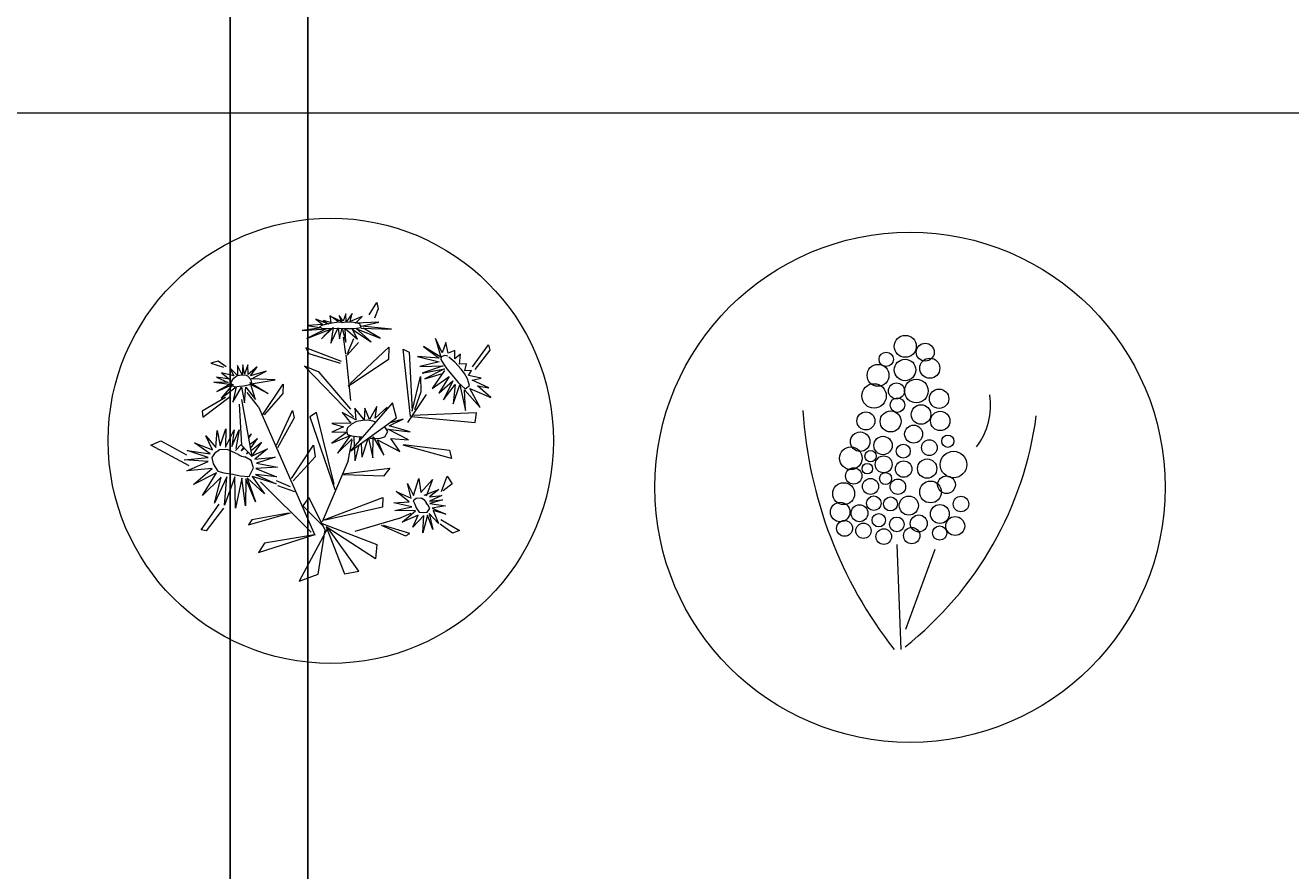
# Model space of a CAD drawing. Units: inches. Extents: x 8049 to 8459, y 820 to 1350.
# Tile 16 of 25: x 8132 to 8165, y 930 to 952. Entities that reach past the tile are written whole.
import ezdxf

# ---------------------------------------------------------------- set-up
doc = ezdxf.new("R2010")
doc.units = ezdxf.units.IN
doc.header["$MEASUREMENT"] = 0
for name, color, linetype, lineweight in [('A-ANNO-DIMS', 2, 'Continuous', 18), ('L-PLNT-BEDS', 94, 'Continuous', 18), ('zelen', 69, 'Continuous', 13)]:
    doc.layers.add(name, color=color, linetype=linetype, lineweight=lineweight)
doc.styles.get("Standard").update_dxf_attribs({"font": 'arial.ttf'})
doc.dimstyles.get("Standard").update_dxf_attribs({"dimtxt": 0.18, "dimasz": 0.18, "dimexe": 0.18, "dimexo": 0.0625, "dimgap": 0.09, "dimtad": 0, "dimtih": 1, "dimtoh": 1, "dimdec": 4, "dimzin": 0, "dimdsep": 46, "dimtxsty": 'Standard', "dimcen": 0.09, "dimadec": 0, "dimazin": 0, "dimtfac": 1, "dimtdec": 4, "dimtofl": 0, "dimtmove": 0, "dimatfit": 3, "dimfxl": 1, "dimtolj": 1, "dimtzin": 0, "dimarcsym": 0})

# ---------------------------------------------------------------- blocks, each defined once
blk = doc.blocks.new('z_07')
for p, q in [((33.4, 283.2), (27.9, 266.9)), ((34.5, 265), (33.4, 283.2)), ((47.8, 284), (34.5, 265)), ((43.1, 265.9), (47.8, 284)), ((85.3, 280.8), (103, 308.6)), ((105.8, 294.2), (97.8, 273.4)), ((103, 308.6), (105.8, 294.2)), ((-17.8, 259.4), (-52, 257.4)), ((-52, 257.4), (-21, 251.8)), ((-33.4, 271.7), (-17.8, 259.4)), ((-5.4, 260.2), (-33.4, 271.7)), ((-17.3, 268.5), (-5.4, 260.2)), ((0.4, 263.9), (-17.3, 268.5)), ((-2, 279), (0.4, 263.9)), ((16.1, 266.2), (-2, 279)), ((6.4, 274.5), (16.1, 266.2)), ((23.4, 266.3), (6.4, 274.5)), ((19, 279.6), (23.4, 266.3)), ((27.9, 266.9), (19, 279.6)), ((70.3, 277.4), (43.1, 265.9)), ((55.3, 262.3), (70.3, 277.4)), ((107.1, 264.9), (55.3, 262.3)), ((68.5, 256.1), (107.1, 264.9)), ((135.2, 249.3), (68.5, 256.1)), ((-21, 251.8), (-63.9, 246.3)), ((-63.9, 246.3), (-10.6, 249.9)), ((-10.6, 249.9), (-53.8, 228)), ((-53.8, 228), (-0.5, 249)), ((-20.7, 227.5), (5.4, 252.6)), ((-0.5, 249), (-20.7, 227.5)), ((5.4, 252.6), (-0.2, 218.2)), ((-0.2, 218.2), (16.1, 251.8)), ((16.1, 251.8), (19.1, 227.4)), ((19.1, 227.4), (25, 251.4)), ((25, 251.4), (33.2, 219.8)), ((33.5, 194.3), (28.4, 231.3)), ((31.7, 250.6), (59.3, 226.6)), ((33.2, 219.8), (31.7, 250.6)), ((37.5, 194.8), (51.1, 228.1)), ((48.1, 248.2), (90.3, 221.2)), ((59.3, 226.6), (48.1, 248.2)), ((57.3, 249.7), (110, 229.2)), ((90.3, 221.2), (57.3, 249.7)), ((67.6, 251), (135.2, 249.3)), ((110, 229.2), (72.3, 251.5)), ((234, 228.4), (245.3, 186.3)), ((248.2, 196), (234, 228.4)), ((-56, 207.7), (-48.9, 194.5)), ((23.9, 176.8), (-56, 207.7)), ((61.7, 219.6), (36.6, 191.4)), ((43.1, 127.7), (129.4, 208.7)), ((129.4, 208.7), (129.1, 181.5)), ((161.2, 204.4), (175.2, 197.9)), ((177.8, 54.5), (161.2, 204.4)), ((175.2, 197.9), (181.3, 66.4)), ((207.2, 210.7), (242, 184.3)), ((245.3, 186.3), (207.2, 210.7)), ((256.8, 219), (248.2, 196)), ((261.8, 195.5), (256.8, 219)), ((276.9, 201.7), (261.8, 195.5)), ((276.6, 182.8), (276.9, 201.7)), ((316.3, 165), (351.8, 213.8)), ((354.7, 202.6), (321.1, 159.3)), ((351.8, 213.8), (354.7, 202.6)), ((-251.2, 177.7), (-267.6, 173.3)), ((-267.6, 173.3), (-239.8, 164.3)), ((-233.4, 165.2), (-251.2, 177.7)), ((-196.5, 169.7), (-197.8, 147.3)), ((-192.3, 148.3), (-196.5, 169.7)), ((-48.9, 194.5), (20.9, 173)), ((33.4, 191.9), (44, 90.1)), ((129.1, 181.5), (39.1, 121.3)), ((193.5, 188), (242.1, 176.2)), ((242, 184.3), (193.5, 188)), ((242.1, 176.2), (198.4, 166.1)), ((246.2, 187.2), (245.4, 181.5)), ((245.4, 181.5), (251.2, 171.8)), ((254.4, 190.4), (246.2, 187.2)), ((251.2, 171.8), (258.8, 160.8)), ((261.3, 189.2), (254.4, 190.4)), ((277.1, 175.7), (263.7, 186.3)), ((289.7, 193.6), (276.6, 182.8)), ((290.7, 160), (277.1, 175.7)), ((287, 171.3), (289.7, 193.6)), ((302.8, 171.8), (287, 171.3)), ((299, 156), (302.8, 171.8)), ((-255.4, 142.2), (-228.7, 129.8)), ((-226, 137.3), (-255.4, 142.2)), ((-243.6, 151.8), (-226, 137.3)), ((-216.2, 145.1), (-243.6, 151.8)), ((-225.7, 163.4), (-216.2, 145.1)), ((-208.5, 145.4), (-225.7, 163.4)), ((-208.7, 144.6), (-219.5, 136.6)), ((-198.7, 146.1), (-208.7, 144.6)), ((-207.9, 168.2), (-208.5, 145.4)), ((-197.8, 147.3), (-207.9, 168.2)), ((-188, 145.4), (-198.7, 146.1)), ((-185.4, 169.2), (-192.3, 148.3)), ((-185.1, 144.1), (-188, 145.4)), ((-184.1, 147.7), (-185.4, 169.2)), ((-179.1, 137.8), (-185.1, 144.1)), ((-164.3, 164.9), (-184.1, 147.7)), ((-179.3, 144.6), (-164.3, 164.9)), ((-144.4, 155), (-179.3, 144.6)), ((-177.3, 138.3), (-144.4, 155)), ((-58.7, 166.4), (50.5, 53.3)), ((-25.8, 153.4), (-58.7, 166.4)), ((44.9, 70.5), (-25.8, 153.4)), ((181.3, 66.4), (199.9, 143.5)), ((198.4, 166.1), (251.1, 167.3)), ((199.9, 143.5), (200.9, 108.9)), ((251.1, 167.3), (203.7, 151)), ((203.7, 151), (254, 160.4)), ((254, 160.4), (209.5, 138.3)), ((209.5, 138.3), (249.1, 150.4)), ((253.9, 156.5), (226.3, 116.7)), ((226.3, 116.7), (263.8, 143.7)), ((263.8, 143.7), (241.3, 106.4)), ((258.8, 160.8), (271.1, 146.1)), ((271.1, 146.1), (284.2, 130.2)), ((298.2, 149.9), (290.7, 160)), ((305.4, 138.6), (298.2, 149.9)), ((314, 156.8), (299, 156)), ((307.2, 145.4), (314, 156.8)), ((335.8, 139.8), (307.2, 145.4)), ((-260.9, 130.5), (-225.2, 126.2)), ((-228.7, 129.8), (-260.9, 130.5)), ((-254.6, 110.2), (-218.2, 126.3)), ((-225.2, 126.2), (-254.6, 110.2)), ((-218.2, 126.3), (-244.5, 95.4)), ((-244.5, 95.4), (-211, 120.2)), ((-219.5, 136.6), (-223.8, 129.5)), ((-223.8, 129.5), (-220.3, 123.5)), ((-220.3, 123.5), (-214.4, 120.6)), ((-211, 120.2), (-218.7, 86)), ((-218.7, 86), (-199, 119.8)), ((-214.4, 120.6), (-204.4, 121.7)), ((-204.4, 121.7), (-194.8, 122.3)), ((-199, 119.8), (-192.3, 84.8)), ((-194.8, 122.3), (-183.9, 124.5)), ((-192.3, 84.8), (-189.8, 119.4)), ((-189.8, 119.4), (-168.3, 91.9)), ((-183.9, 124.5), (-175.3, 127)), ((-179.8, 129.8), (-139.5, 105.2)), ((-168.3, 91.9), (-179.8, 129.8)), ((-177.1, 133.3), (-179.1, 137.8)), ((-177.5, 126.2), (-176.4, 128.6)), ((-139.5, 105.2), (-177.5, 124.5)), ((-124, 136.2), (-177.3, 138.3)), ((-176.4, 128.6), (-177.1, 133.3)), ((-173.3, 127.9), (-124, 136.2)), ((-153, 56.3), (-106.3, 126)), ((-106.3, 126), (-106.9, 105.8)), ((241.3, 106.4), (272.2, 133.8)), ((272.2, 133.8), (251.6, 91.4)), ((251.6, 91.4), (277.6, 125.4)), ((277.6, 125.4), (273.2, 82.7)), ((273.2, 82.7), (288.2, 124.6)), ((284.2, 130.2), (299.9, 116.2)), ((288.2, 124.6), (300.3, 67.6)), ((298.3, 113.8), (333.6, 74.1)), ((300.3, 67.6), (298.3, 113.8)), ((299.9, 116.2), (309.5, 123)), ((309.5, 123), (305.4, 138.6)), ((310, 116.8), (357.4, 96.4)), ((333.6, 74.1), (310, 116.8)), ((315.5, 135.5), (335.8, 139.8)), ((352.4, 118.2), (315.5, 135.5)), ((327.7, 122.6), (352.4, 118.2)), ((357.4, 96.4), (327.7, 122.6)), ((-235.3, 96.4), (-287.1, 65.9)), ((-285.8, 52.5), (-224.8, 98.6)), ((-175.3, -35.1), (-198.7, 92.4)), ((-161, 75.8), (-186.5, 108.1)), ((-106.9, 105.8), (-148.5, 57.6)), ((213, 103.6), (171.4, 40.8)), ((200.9, 108.9), (186.6, 68.8)), ((-287.1, 65.9), (-285.8, 52.5)), ((-204.6, 81.4), (-199.5, -9.8)), ((-161, 75.8), (-35.7, -210.4)), ((-121, -10), (-85.7, 67.7)), ((-85.7, 67.7), (-81.5, 51.1)), ((-32.2, 63.2), (-46.9, 53.3)), ((7.2, -97), (-32.2, 63.2)), ((25.4, 62.8), (44.7, 39.2)), ((55.8, 46.8), (25.4, 62.8)), ((137.7, 84.7), (43.3, -23)), ((53.9, 72.9), (55.8, 46.8)), ((74.4, 46.6), (53.9, 72.9)), ((75.8, 72.7), (74.4, 46.6)), ((86.1, 47.7), (75.8, 72.7)), ((102.6, 76.8), (86.1, 47.7)), ((98.7, 50.4), (102.6, 76.8)), ((125.5, 74.7), (98.7, 50.4)), ((121.6, 66.3), (125.5, 74.7)), ((146.5, 51), (137.7, 84.7)), ((325.5, 62.5), (181.8, 56.3)), ((322.4, 41), (325.5, 62.5)), ((-81.5, 51.1), (-118.8, -15.9)), ((-46.9, 53.3), (9.1, -108.7)), ((44.7, 39.2), (2.2, 38.8)), ((2.2, 38.8), (28.3, 31)), ((28.3, 31), (2.4, 19.3)), ((36.9, 28.9), (34.9, 20.5)), ((46.1, 37.3), (36.9, 28.9)), ((44.9, -22.6), (146.5, 51)), ((57.5, 43.2), (46.1, 37.3)), ((71.6, 45.6), (57.5, 43.2)), ((83, 45.7), (71.6, 45.6)), ((93.9, 43.8), (83, 45.7)), ((99.9, 41.6), (93.9, 43.8)), ((119.3, 31.3), (122.2, 29)), ((127.4, 21), (122.2, 29)), ((130.2, 33), (162.1, 48.8)), ((177.4, 19.7), (130.2, 33)), ((132.6, 41), (162.1, 48.8)), ((179.2, 54.2), (322.4, 41)), ((-278.8, 11), (-256.7, -14.8)), ((-264.2, -20.1), (-278.8, 11)), ((-256.7, -14.8), (-253.9, 22.7)), ((-253.9, 22.7), (-246.6, -11.2)), ((-246.6, -11.2), (-233.9, 26.9)), ((-233.9, 26.9), (-234.7, -14.3)), ((-234.7, -14.3), (-215.8, 24.7)), ((-215.8, 24.7), (-221.2, -12.7)), ((-221.2, -12.7), (-204.3, 24.2)), ((-204.3, 24.2), (-211.6, -17)), ((-183.3, 9.2), (-177.1, 15.7)), ((-182.9, 5.9), (-177.1, 15.7)), ((-179.2, -7.1), (-163.5, 4.7)), ((-177.8, -14.9), (-163.5, 4.7)), ((37.5, 20.3), (2.2, -5.3)), ((2.2, -5.3), (43.4, 11.4)), ((2.4, 19.3), (37.5, 20.3)), ((43.4, 11.4), (15.2, -28)), ((15.2, -28), (47.4, 4.5)), ((34.9, 20.5), (37.2, 13.9)), ((37.2, 13.9), (45.9, 11)), ((39.1, -45), (47.8, 1.4)), ((45.9, 11), (63.1, 9.1)), ((52.7, -13), (51.9, 8.7)), ((69.3, 8.1), (63.1, 9.1)), ((64.2, 2), (65.3, 8.2)), ((65.3, 8.2), (66.2, 4.8)), ((82.3, 4.4), (69.2, -36.7)), ((84.4, 6), (93.9, -38.4)), ((87.1, 6.1), (91, 5.8)), ((91, 5.8), (107, 4.7)), ((93.9, -38.4), (94.9, 9.1)), ((94.9, 9.1), (118.4, -31.9)), ((103.9, 1.8), (153.8, -23.7)), ((118.4, -31.9), (103.9, 1.8)), ((107, 4.7), (120.6, 8.6)), ((120.6, 8.6), (127.4, 21)), ((127.5, 26.1), (177.4, 19.7)), ((173.6, 2.2), (127.5, 26.1)), ((133.7, 4.9), (173.6, 2.2)), ((153.8, -23.7), (133.7, 4.9)), ((-401.9, -9.6), (-379.5, -0.2)), ((-316.3, -55.6), (-401.9, -9.6)), ((-379.5, -0.2), (-321.8, -31.6)), ((-320.8, -21.7), (-269.2, -29.5)), ((-273.5, -37.2), (-320.8, -21.7)), ((-304.1, -4.5), (-264.2, -20.1)), ((-269.2, -29.5), (-304.1, -4.5)), ((-199.2, -7.5), (-212.9, -21.9)), ((-195.5, -15.5), (-199.7, -22.6)), ((-194, -18.3), (-199.7, -22.6)), ((-199.5, -9.8), (-175.3, -35.1)), ((-185.4, -25.3), (-188.2, -29.1)), ((-185.3, -26.8), (-188.2, -29.1)), ((-177.3, -20.7), (-154.6, -3.3)), ((-154.6, -3.3), (-177, -34.7)), ((-177, -34.7), (-141.4, -17.9)), ((-141.4, -17.9), (-169.7, -41.4)), ((-87.9, -84.4), (-38.6, -9.6)), ((-38.6, -9.6), (-35.2, -35.6)), ((52.9, -17.7), (53.9, -45.1)), ((62.8, -9.7), (53.9, -45.1)), ((67.9, -6), (69.2, -36.7)), ((269.4, -39.7), (161.2, -10.1)), ((162.5, -8), (265, -20.8)), ((265, -20.8), (269.4, -39.7)), ((-327.2, -42.6), (-273.5, -37.2)), ((-273.3, -46.2), (-327.2, -42.6)), ((-321.4, -67.4), (-273.3, -46.2)), ((-169.7, -41.4), (-123.8, -36.5)), ((-123.8, -36.5), (-165.8, -50.2)), ((-165.8, -50.2), (-119, -59.3)), ((-35.2, -35.6), (-84.2, -89.8)), ((39.1, -45), (-19, -181)), ((-264.4, -61.8), (-321.4, -67.4)), ((-306.3, -97.5), (-264.4, -61.8)), ((-254.9, -71.5), (-306.3, -97.5)), ((-286.2, -122.5), (-254.9, -71.5)), ((-244.5, -81.1), (-286.2, -122.5)), ((-232, -80.6), (-259.7, -139.6)), ((-259.7, -139.6), (-244.5, -81.1)), ((-214.2, -80.4), (-237.3, -144.1)), ((-237.3, -144.1), (-232, -80.6)), ((-212.8, -150.3), (-214.2, -80.4)), ((-198.5, -83.3), (-212.8, -150.3)), ((-190.2, -145.4), (-198.5, -83.3)), ((-186.3, -82.5), (-167.7, -136.5)), ((-147.8, -118.8), (-186.3, -82.5)), ((-175.8, -80), (-147.8, -118.8)), ((-121.6, -96.5), (-175.8, -80)), ((-168, -75), (-121.6, -96.5)), ((-120.9, -80.4), (-168, -75)), ((-119, -59.3), (-167.6, -62.1)), ((-167.6, -62.1), (-120.9, -80.4)), ((27.1, -73.7), (132.1, -61.1)), ((117.7, -79.1), (28.4, -76.2)), ((132.1, -61.1), (117.7, -79.1)), ((184.9, -122.5), (196.7, -84.2)), ((196.7, -84.2), (200.9, -115.8)), ((247, -112.9), (259.8, -79.1)), ((259.8, -79.1), (270.8, -96.5)), ((-189.5, -85.3), (-190.2, -145.4)), ((-167.7, -136.5), (-189.5, -85.3)), ((-157.2, -91.9), (-44.1, -203.7)), ((-90.2, -102.6), (-121.5, -89.6)), ((-80.5, -114), (-118, -100.6)), ((171.4, -95.7), (184.9, -122.5)), ((179.1, -127.9), (171.4, -95.7)), ((200.9, -115.8), (227.1, -86.7)), ((208.5, -121.7), (241.2, -108.7)), ((227.1, -86.7), (212.5, -123.9)), ((241.2, -108.7), (219.9, -125.3)), ((270.8, -96.5), (251.1, -111.6)), ((-49.1, -127), (-62.3, -145)), ((-12.6, -198.5), (-49.1, -127)), ((-17.1, -177), (116.1, -126.4)), ((116.1, -126.4), (115.5, -148.1)), ((140.7, -138.3), (175.2, -136.5)), ((180.5, -147.4), (140.7, -138.3)), ((145.9, -113.6), (179.1, -127.9)), ((175.2, -136.5), (145.9, -113.6)), ((219.9, -125.3), (247.4, -121.9)), ((247.4, -121.9), (220.2, -134.6)), ((220.2, -134.6), (249.2, -132)), ((249.2, -132), (220.8, -140.2)), ((220.8, -140.2), (255.6, -145.2)), ((-289.3, -199.2), (-249.4, -141.8)), ((-239.8, -150.1), (-278.3, -200.8)), ((-183.8, -187.5), (-90.1, -161.1)), ((-94.3, -161.3), (-176, -176.8)), ((-62.3, -145), (-16, -191.1)), ((115.5, -148.1), (-12.7, -177.2)), ((142.6, -156), (180.5, -147.4)), ((189.3, -156.2), (142.6, -156)), ((151.6, -173.6), (179.7, -161.5)), ((158.9, -181.7), (189.3, -156.2)), ((194.8, -166.3), (158.9, -181.7)), ((183.3, -192.9), (194.8, -166.3)), ((207.6, -167.1), (183.3, -192.9)), ((215.9, -165.8), (205.3, -205.2)), ((205.3, -205.2), (207.6, -167.1)), ((227.9, -197.8), (215.9, -165.8)), ((219.6, -162.5), (227.9, -197.8)), ((240.6, -184.8), (219.6, -162.5)), ((255.6, -145.2), (226.2, -150.6)), ((226.2, -150.6), (256.4, -164)), ((228.7, -155.9), (240.6, -184.8)), ((256.4, -164), (228.7, -155.9)), ((-176, -176.8), (-183.8, -187.5)), ((-6.3, -194.1), (-70.4, -313.3)), ((-19.5, -184.8), (103, -231.9)), ((-10.4, -192.3), (30.8, -297.4)), ((99.4, -263.3), (-10.4, -192.3)), ((62.9, -291.3), (-6.3, -194.1)), ((151.6, -173.6), (53.5, -202.8)), ((112.5, -188.5), (167, -212.2)), ((176.5, -207.3), (117.7, -188.9)), ((271.8, -206.6), (243.8, -186.4)), ((245.2, -175.7), (287.5, -200.6)), ((-278.3, -200.8), (-289.3, -199.2)), ((-161, -249.4), (-37.6, -210)), ((-36.1, -210), (-148.2, -228.8)), ((-28, -297.6), (-12.6, -198.5)), ((167, -212.2), (176.5, -207.3)), ((287.5, -200.6), (271.8, -206.6)), ((-148.2, -228.8), (-161, -249.4)), ((103, -231.9), (99.4, -263.3)), ((-70.4, -313.3), (-28, -297.6)), ((30.8, -297.4), (62.9, -291.3))]:
    blk.add_line(p, q)
for points in [[(26.3, 263.3), (22.9, 264.5), (12.8, 264.3), (2.9, 262.7), (-9.7, 260.6), (-20.2, 257.5), (-25.1, 254.7), (-20.2, 251.3), (-1.3, 250.6), (16.7, 251.1), (38.2, 250.3), (52.3, 250.3), (67.9, 252.7), (64.7, 261.3), (50.6, 264.3), (36.5, 264.6), (22.8, 262.9)], [(-211.4, -28.6), (-222.1, -23.5), (-231.1, -19.5), (-248.3, -20.6), (-259.5, -28.3), (-265.7, -37.4), (-262.3, -51.8), (-252.4, -67.8), (-238.9, -71.3), (-218.5, -74.3), (-202.3, -78), (-182.1, -79.6), (-172.2, -60.6), (-177.8, -44.4), (-191.8, -35.5)], [(-211.4, -28.6), (-208.4, -29.2), (-206.4, -30.7), (-204.3, -31.6), (-202.2, -33.1), (-199.4, -34.2), (-195.7, -35.1), (-191.8, -35.8), (-191.8, -35.5)], [(214.6, -141.2), (213.8, -137.6), (210, -133.3), (202.5, -128.4), (190.3, -129), (183.7, -134.2), (187.4, -141.4), (190.6, -149.7), (197.3, -159.1), (207.6, -160.4), (215.4, -159.3), (220.7, -151.3), (216.9, -142.9), (213.1, -138.2)]]:
    blk.add_lwpolyline(points)
blk.add_circle((0, 0), 496.9)
blk = doc.blocks.new('z_06')
for p, q in [((-26, -111.8), (-18.2, -317.4)), ((48.7, -121.5), (-8.6, -278.6))]:
    blk.add_line(p, q)
for centre, radius in [((0, 0), 499.1), ((-9.3, 275.8), 21.5), ((29.8, 264.3), 17.5), ((-46.5, 250.4), 14), ((-9.7, 229.6), 21.1), ((38.7, 232.9), 19.7), ((-62.5, 219), 21.4), ((-70.3, 178.8), 23.9), ((-26.4, 188.5), 15.7), ((12.3, 188.5), 23.2), ((-24.6, 160.8), 14.2), ((56.9, 173.3), 19), ((-37.9, 128.9), 20.5), ((21.6, 142.3), 19.1), ((59.1, 129.8), 19), ((-86.3, 129.8), 17.6), ((-97.5, 89.2), 19.1), ((-52.8, 81.8), 18), ((7.1, 104), 17.6), ((74, 90.1), 12), ((-115.7, 56.8), 22.2), ((-13.1, 70.7), 13.7), ((37.9, 77.6), 15.4), ((-77, 60.9), 11.1), ((-51.5, 44.9), 16.6), ((-12.5, 35.6), 16.1), ((33.5, 36.5), 18.9), ((85.2, 44.4), 26), ((-110.1, 22.2), 15.9), ((-83.5, 36.4), 10.2), ((-47.9, 17.1), 11.7), ((-129.8, -12.5), 21.4), ((-77.3, 1.7), 15.7), ((-23.7, 1), 15.1), ((40.2, -9.2), 21.3), ((71.4, 5.1), 17.3), ((-70.8, -31.2), 14.2), ((-38.2, -32.7), 13.7), ((-2.3, -35.8), 18.7), ((99.7, -32.8), 15.2), ((-136.5, -48.5), 19.1), ((-98.8, -50.8), 16.5), ((58.4, -52.2), 18.5), ((-128, -80.4), 15.5), ((-91.1, -85.1), 15), ((-61.1, -64.4), 13.1), ((-25.8, -72.6), 14.4), ((17.1, -70.7), 16.5), ((88.5, -75.8), 18.5), ((-51.3, -96.5), 15.3), ((3.4, -94.5), 16), ((58, -89.6), 14)]:
    blk.add_circle(centre, radius)
for centre, radius, start, end in [((21.1, 161.1), 136.5, 323.03, 8.2301), ((631.6, 203.5), 842.7, 183.6263, 218.177), ((-440.2, 231.1), 693.3, 308.3911, 352.4108)]:
    blk.add_arc(centre, radius, start, end)
blk = doc.blocks.new('*D58')
at = {"layer": 'A-ANNO-DIMS', "color": 0, "lineweight": -2, "transparency": 16777216}
for p, q in [((8139.397, 1162.808), (8139.397, 820.091)), ((8175.397, 1162.808), (8175.397, 820.091)), ((8139.577, 820.271), (8157.179, 820.271)), ((8175.217, 820.271), (8157.616, 820.271))]:
    blk.add_line(p, q, dxfattribs=at)
at = {"layer": 'A-ANNO-DIMS', "color": 0, "transparency": 16777216}
for points in [[(8139.577, 820.301), (8139.577, 820.241), (8139.397, 820.271)], [(8175.217, 820.301), (8175.217, 820.241), (8175.397, 820.271)]]:
    blk.add_solid(points, dxfattribs=at)
at = {"layer": 'Defpoints', "color": 0, "transparency": 16777216}
for p in [(8139.397, 1162.871), (8175.397, 1162.871), (8175.397, 820.271)]:
    blk.add_point(p, dxfattribs=at)
at = {"layer": 'A-ANNO-DIMS', "color": 0, "transparency": 16777216, "insert": (8157.397, 820.271), "char_height": 0.18, "attachment_point": 5}
blk.add_mtext('\\A1;36', dxfattribs=at)
blk = doc.blocks.new('*D70')
at = {"layer": 'A-ANNO-DIMS', "color": 0, "lineweight": -2, "transparency": 16777216}
for p, q in [((8083.397, 1045.808), (8083.397, 820.091)), ((8137.397, 1045.808), (8137.397, 820.091)), ((8083.577, 820.271), (8110.179, 820.271)), ((8137.217, 820.271), (8110.616, 820.271))]:
    blk.add_line(p, q, dxfattribs=at)
at = {"layer": 'A-ANNO-DIMS', "color": 0, "transparency": 16777216}
for points in [[(8083.577, 820.301), (8083.577, 820.241), (8083.397, 820.271)], [(8137.217, 820.301), (8137.217, 820.241), (8137.397, 820.271)]]:
    blk.add_solid(points, dxfattribs=at)
at = {"layer": 'Defpoints', "color": 0, "transparency": 16777216}
for p in [(8083.397, 1045.871), (8137.397, 1045.871), (8083.397, 820.271)]:
    blk.add_point(p, dxfattribs=at)
at = {"layer": 'A-ANNO-DIMS', "color": 0, "transparency": 16777216, "insert": (8110.397, 820.271), "char_height": 0.18, "attachment_point": 5}
blk.add_mtext('\\A1;54', dxfattribs=at)
blk = doc.blocks.new('*D76')
at = {"layer": 'A-ANNO-DIMS', "color": 0, "lineweight": -2, "transparency": 16777216}
for p, q in [((8083.397, 1054.808), (8083.397, 820.091)), ((8299.397, 1054.808), (8299.397, 820.091)), ((8083.577, 820.271), (8191.107, 820.271)), ((8299.217, 820.271), (8191.688, 820.271))]:
    blk.add_line(p, q, dxfattribs=at)
at = {"layer": 'A-ANNO-DIMS', "color": 0, "transparency": 16777216}
for points in [[(8083.577, 820.301), (8083.577, 820.241), (8083.397, 820.271)], [(8299.217, 820.301), (8299.217, 820.241), (8299.397, 820.271)]]:
    blk.add_solid(points, dxfattribs=at)
at = {"layer": 'Defpoints', "color": 0, "transparency": 16777216}
for p in [(8083.397, 1054.871), (8299.397, 1054.871), (8299.397, 820.271)]:
    blk.add_point(p, dxfattribs=at)
at = {"layer": 'A-ANNO-DIMS', "color": 0, "transparency": 16777216, "insert": (8191.397, 820.271), "char_height": 0.18, "attachment_point": 5}
blk.add_mtext('\\A1;216', dxfattribs=at)
blk = doc.blocks.new('*D88')
at = {"layer": 'A-ANNO-DIMS', "color": 0, "lineweight": -2, "transparency": 16777216}
for p, q in [((8083.397, 1162.808), (8083.397, 820.091)), ((8139.397, 1162.808), (8139.397, 820.091)), ((8083.577, 820.271), (8111.179, 820.271)), ((8139.217, 820.271), (8111.616, 820.271))]:
    blk.add_line(p, q, dxfattribs=at)
at = {"layer": 'A-ANNO-DIMS', "color": 0, "transparency": 16777216}
for points in [[(8083.577, 820.301), (8083.577, 820.241), (8083.397, 820.271)], [(8139.217, 820.301), (8139.217, 820.241), (8139.397, 820.271)]]:
    blk.add_solid(points, dxfattribs=at)
at = {"layer": 'Defpoints', "color": 0, "transparency": 16777216}
for p in [(8083.397, 1162.871), (8139.397, 1162.871), (8139.397, 820.271)]:
    blk.add_point(p, dxfattribs=at)
at = {"layer": 'A-ANNO-DIMS', "color": 0, "transparency": 16777216, "insert": (8111.397, 820.271), "char_height": 0.18, "attachment_point": 5}
blk.add_mtext('\\A1;56', dxfattribs=at)

msp = doc.modelspace()

# ---------------------------------------------------------------- linework, layer by layer
at = {"layer": 'L-PLNT-BEDS'}
msp.add_line((8083.3974, 949.8706), (8197.3974, 949.8706), dxfattribs=at)

# ---------------------------------------------------------------- block references
at = {"layer": 'zelen'}
for name, p, xscale, yscale, zscale in [('z_07', (8139.9895, 941.4066), 0.0115605630918543, 0.0115605630918543, 0.0115605630918543), ('z_06', (8154.9319, 940.2061), 0.0131883500742978, 0.0131883500742978, 0.0131883500742978)]:
    msp.add_blockref(name, p, dxfattribs=dict(at, xscale=xscale, yscale=yscale, zscale=zscale))

# ---------------------------------------------------------------- dimensions: what is measured, and where the dimension line sits
at = {"layer": 'A-ANNO-DIMS'}
for base, p1, p2, picture, middle in [((8139.3974, 820.2706), (8083.3974, 1162.8706), (8139.3974, 1162.8706), '*D88', (8111.3974, 820.2706)), ((8175.3974, 820.2706), (8139.3974, 1162.8706), (8175.3974, 1162.8706), '*D58', (8157.3974, 820.2706)), ((8299.3974, 820.2706), (8083.3974, 1054.8706), (8299.3974, 1054.8706), '*D76', (8191.3974, 820.2706)), ((8083.3974, 820.2706), (8137.3974, 1045.8706), (8083.3974, 1045.8706), '*D70', (8110.3974, 820.2706))]:
    dim = msp.add_linear_dim(base=base, p1=p1, p2=p2, dimstyle='Standard', override={"dimdec": 0, "dimlfac": 1, "dimrnd": 0, "dimzin": 0, "dimdsep": 46, "dimlunit": 2}, dxfattribs=at)
    dim.commit()
    dim.dimension.update_dxf_attribs({"geometry": picture, "text_midpoint": middle})

doc.saveas('drawing.dxf')
